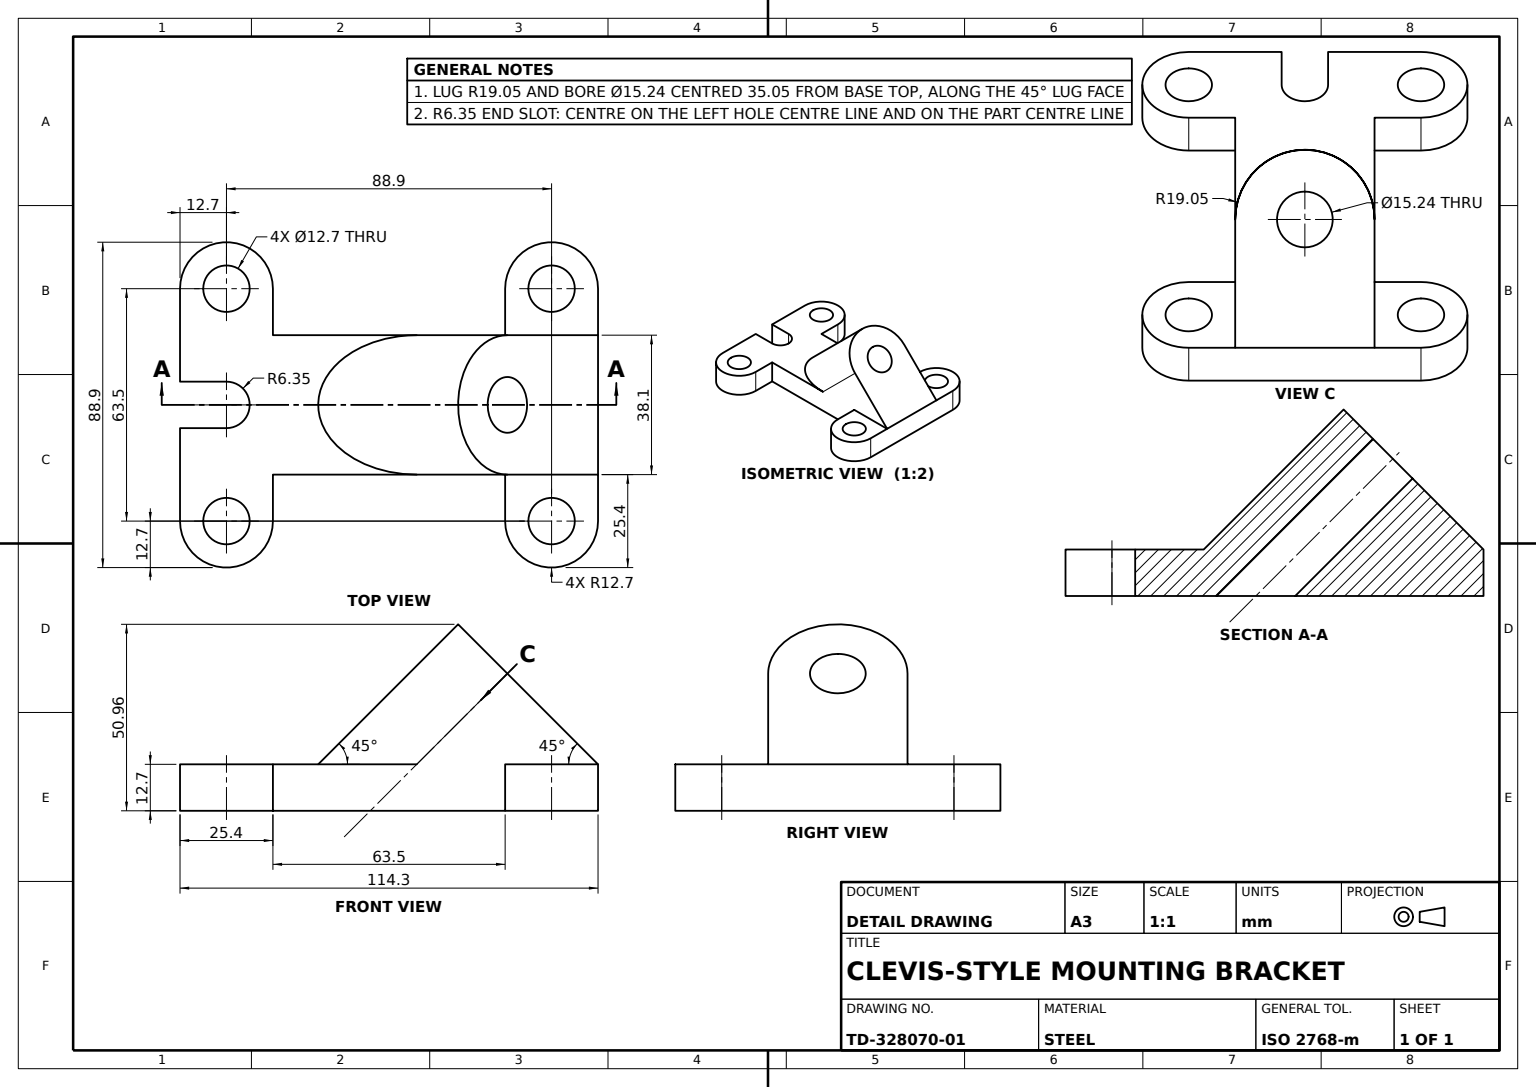
from build123d import *

# Parameters (mm, degrees)
BASE_PLATE_SKETCH_W     = 38.1
BASE_PLATE_SKETCH_H     = 63.5
BASE_PLATE_DEPTH        = 12.7
MOUNTING_HOLES_SKETCH_R = 6.35
MOUNTING_HOLES_DEPTH    = 112.622813528
INCLINED_LUG_REACH      = 102.603
LUG_BORE_REACH          = 102.603
LUG_BORE_SKETCH_R       = 7.62


with BuildPart() as part:
    # Base Plate Sketch → Base Plate (new body)
    with BuildSketch(Plane(origin=(0, 0, 0), x_dir=(1, 0, 0), z_dir=(0, 1, 0))):
        with BuildLine():
            Line((31.75, 12.7), (-31.75, 12.7))
            ThreePointArc((-31.75, 12.7), (-44.45, 0), (-31.75, -12.7))
            Line((-31.75, -12.7), (31.75, -12.7))
            ThreePointArc((31.75, -12.7), (44.45, 0), (31.75, 12.7))
        make_face()
        with Locations((0, -44.45)):
            Rectangle(BASE_PLATE_SKETCH_W, BASE_PLATE_SKETCH_H)
        with BuildLine():
            Line((31.75, -76.2), (-31.75, -76.2))
            ThreePointArc((-31.75, -76.2), (-44.45, -88.9), (-31.75, -101.6))
            Line((-31.75, -101.6), (31.75, -101.6))
            ThreePointArc((31.75, -101.6), (44.45, -88.9), (31.75, -76.2))
        make_face()
    extrude(amount=BASE_PLATE_DEPTH)

    # Mounting Holes Sketch → Mounting Holes (cut, through all)
    with BuildSketch(Plane(origin=(0, 12.7, 0), x_dir=(1, 0, 0), z_dir=(0, 1, 0))):
        with Locations(Location((-31.75, 0, 0), (0, 0, 270))):
            Circle(MOUNTING_HOLES_SKETCH_R)
        with Locations(Location((31.75, 0, 0), (0, 0, 270))):
            Circle(MOUNTING_HOLES_SKETCH_R)
        with Locations(Location((-31.75, -88.9, 0), (0, 0, 270))):
            Circle(MOUNTING_HOLES_SKETCH_R)
        with Locations(Location((31.75, -88.9, 0), (0, 0, 270))):
            Circle(MOUNTING_HOLES_SKETCH_R)
        with BuildLine():
            Line((-6.35, 0), (-6.35, 12.7))
            Line((-6.35, 12.7), (6.35, 12.7))
            Line((6.35, 12.7), (6.35, 0))
            ThreePointArc((6.35, 0), (0, -6.35), (-6.35, 0))
        make_face()
    extrude(amount=-MOUNTING_HOLES_DEPTH, mode=Mode.SUBTRACT)

    # Inclined Lug Sketch → Inclined Lug (add, up to next)
    with BuildSketch(Plane(origin=(0, 57.15, 57.15), x_dir=(-1, 0, 0), z_dir=(0, 0.7071067811865488, 0.7071067811865464)), mode=Mode.PRIVATE) as inclined_lug_sk1:
        with BuildLine():
            Line((-19.05, 62.861792847), (19.05, 62.861792847))
            Line((19.05, 62.861792847), (19.05, 27.809792847))
            ThreePointArc((19.05, 27.809792847), (0, 8.759792847), (-19.05, 27.809792847))
            Line((-19.05, 27.809792847), (-19.05, 62.861792847))
        make_face()
    inclined_lug_tool1 = extrude(inclined_lug_sk1.sketch, amount=-INCLINED_LUG_REACH, mode=Mode.PRIVATE) - part.part
    add(inclined_lug_tool1.solids().sort_by_distance((0, 30.51036, 83.78964))[0])

    # Lug Bore: up to this plane
    lug_bore_end = Plane(origin=(0, 0, 0), z_dir=(0, 1, 0))
    # Lug Bore Sketch → Lug Bore (cut, up to the surface)
    with BuildSketch(Plane(origin=(0, 57.15, 57.15), x_dir=(1, 0, 0), z_dir=(0, 0.7071067811865487, 0.7071067811865465)), mode=Mode.PRIVATE) as lug_bore_sk1:
        with Locations(Location((0, -27.809792847, 0), (0, 0, 270))):
            Circle(LUG_BORE_SKETCH_R)
    lug_bore_tool1 = split(extrude(lug_bore_sk1.sketch, amount=-LUG_BORE_REACH, mode=Mode.PRIVATE), bisect_by=lug_bore_end, keep=Keep.BOTH, mode=Mode.PRIVATE)
    add(lug_bore_tool1.solids().sort_by_distance((0, 37.485507, 76.814493))[0], mode=Mode.SUBTRACT)


solid = part.part
